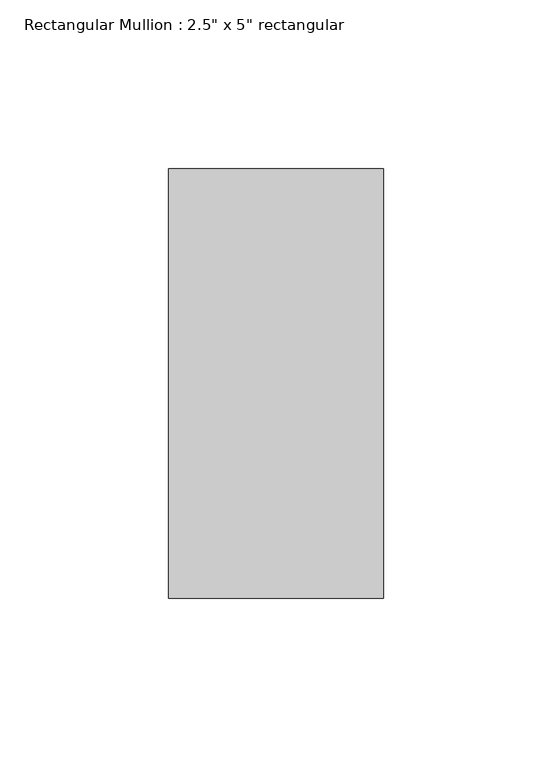
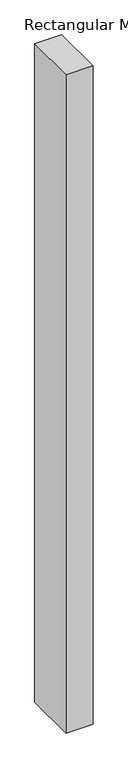
"""IFC4 building model written with IfcOpenShell, lengths in millimetres: member geometry."""

from ifc_helpers import new_model, si_unit, frame, origin, place, context, project, spatial, polyline, outline, extrude, source, transform, mapped, element, save


def member_2f7568ae(model_context):
    return source(origin(), model_context, "Body", "SweptSolid", [
        extrude(outline(polyline([(31.75, 63.5), (31.75, -63.5), (-31.75, -63.5), (-31.75, 63.5), (31.75, 63.5)])), frame((0.0, 0.0, -1634.3549218), z_axis=(0.0, 0.0, 1.0), x_axis=(1.0, 0.0, 0.0)), (0.0, 0.0, 1.0), 1634.3549218),
    ])


if __name__ == "__main__":
    model = new_model("IFC4")
    model_context = context("Model", 3, world=origin())
    ifc_project = project(units=[si_unit("LENGTHUNIT", "METRE", prefix="MILLI")], contexts=[model_context])
    site = spatial("IfcSite", under=ifc_project)
    building = spatial("IfcBuilding", under=site)
    placement = place(None, origin())
    member_shape = member_2f7568ae(model_context)
    element("IfcMember", 1, ObjectType="Rectangular Mullion : 2.5\" x 5\" rectangular", at=placement, inside=building, context=model_context, shape_type="MappedRepresentation", body=[
        mapped(member_shape, transform((0.0, 0.0, 0.0), x_axis=(1.0, 0.0, 0.0), y_axis=(0.0, 1.0, 0.0), z_axis=(0.0, 0.0, 1.0))),
    ])
    save(model, "model.ifc")

# Revit data of these elements
# Type "Rectangular Mullion : 2.5\" x 5\" rectangular"
#   built-in parameter 1007304 = 0.416667 (stored number, unit not read)
#   built-in parameter 1007301 = 0.104167 (stored number, unit not read)
#   built-in parameter 1007300 = 0.104167 (stored number, unit not read)
# Element 1 (IfcMember, "Rectangular Mullion : 2.5\" x 5\" rectangular")
#   Materials on its faces: "Aluminum"
# Materials
#   "Aluminum": class "Metal", colour RGB 247 247 247, transparency 0, Description = "Aluminum 6061", Cost = 0
